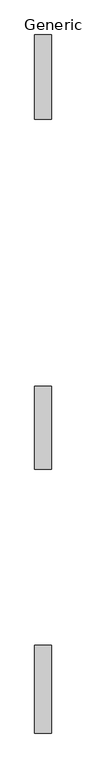
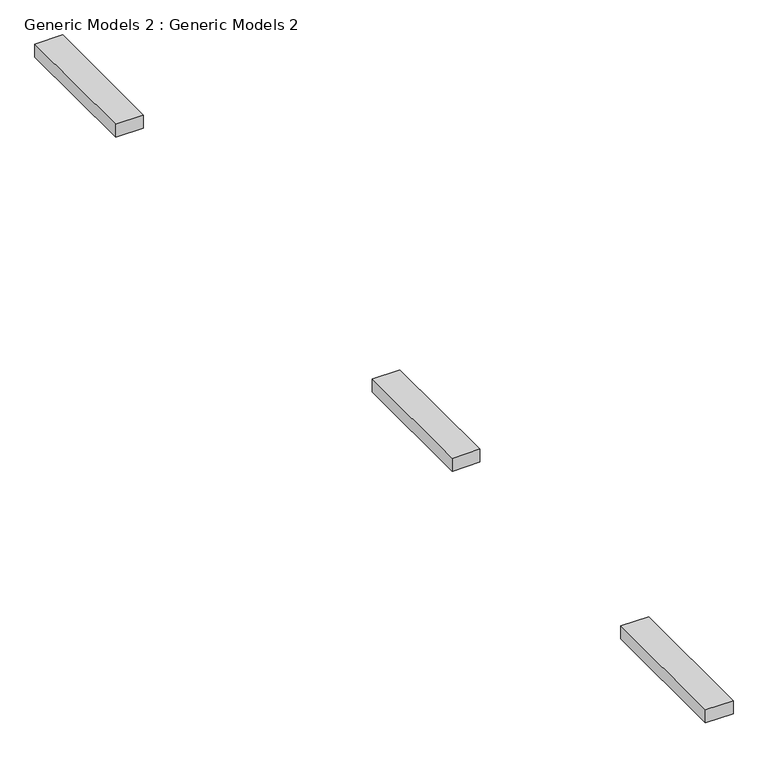
"""IFC4 building model written with IfcOpenShell, lengths in millimetres: proxy geometry, Generic Models 2 : Generic Models 2."""

from ifc_helpers import new_model, si_unit, frame, origin, place, context, project, spatial, polyline, outline, extrude, source, transform, mapped, element, save


def generic_models_2_generic_models_2_71c639ae(model_context):
    return source(origin(), model_context, "Body", "SweptSolid", [
        extrude(outline(polyline([(-3150.8771954, -3782.7227897), (-3150.8771954, -5395.5736261), (-3455.6771954, -5395.5736261), (-3455.6771954, -3782.7227897), (-3150.8771954, -3782.7227897)])), frame((0.0, 0.0, 2260.6), z_axis=(0.0, 0.0, 1.0), x_axis=(1.0, 0.0, 0.0)), (0.0, 0.0, 1.0), 152.4),
        extrude(outline(polyline([(-3150.8771954, 963.3008967), (-3150.8771954, -560.9825441), (-3455.6771954, -560.9825441), (-3455.6771954, 963.3008967), (-3150.8771954, 963.3008967)])), frame((0.0, 0.0, 2260.6), z_axis=(0.0, 0.0, 1.0), x_axis=(1.0, 0.0, 0.0)), (0.0, 0.0, 1.0), 152.4),
        extrude(outline(polyline([(-3150.8771954, 7403.0267346), (-3150.8771954, 5859.3819001), (-3455.6771954, 5859.3819001), (-3455.6771954, 7403.0267346), (-3150.8771954, 7403.0267346)])), frame((0.0, 0.0, 2260.6), z_axis=(0.0, 0.0, 1.0), x_axis=(1.0, 0.0, 0.0)), (0.0, 0.0, 1.0), 152.4),
    ])


if __name__ == "__main__":
    model = new_model("IFC4")
    model_context = context("Model", 3, world=origin())
    ifc_project = project(units=[si_unit("LENGTHUNIT", "METRE", prefix="MILLI")], contexts=[model_context])
    site = spatial("IfcSite", under=ifc_project)
    building = spatial("IfcBuilding", under=site)
    placement = place(None, origin())
    generic_models_2_generic_models_2_shape = generic_models_2_generic_models_2_71c639ae(model_context)
    element("IfcBuildingElementProxy", 1, Name="Generic Models 2 : Generic Models 2", ObjectType="Generic Models 2 : Generic Models 2", at=placement, inside=building, context=model_context, shape_type="MappedRepresentation", body=[
        mapped(generic_models_2_generic_models_2_shape, transform((0.0, 0.0, 0.0), x_axis=(1.0, 0.0, 0.0), y_axis=(0.0, 1.0, 0.0), z_axis=(0.0, 0.0, 1.0))),
    ])
    save(model, "model.ifc")
